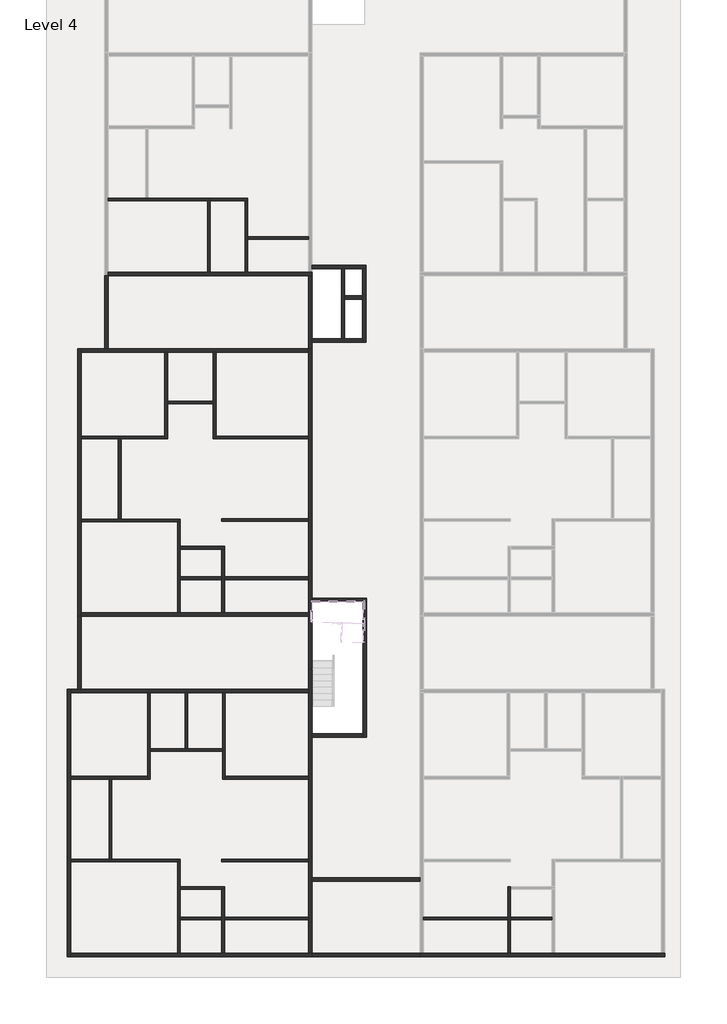
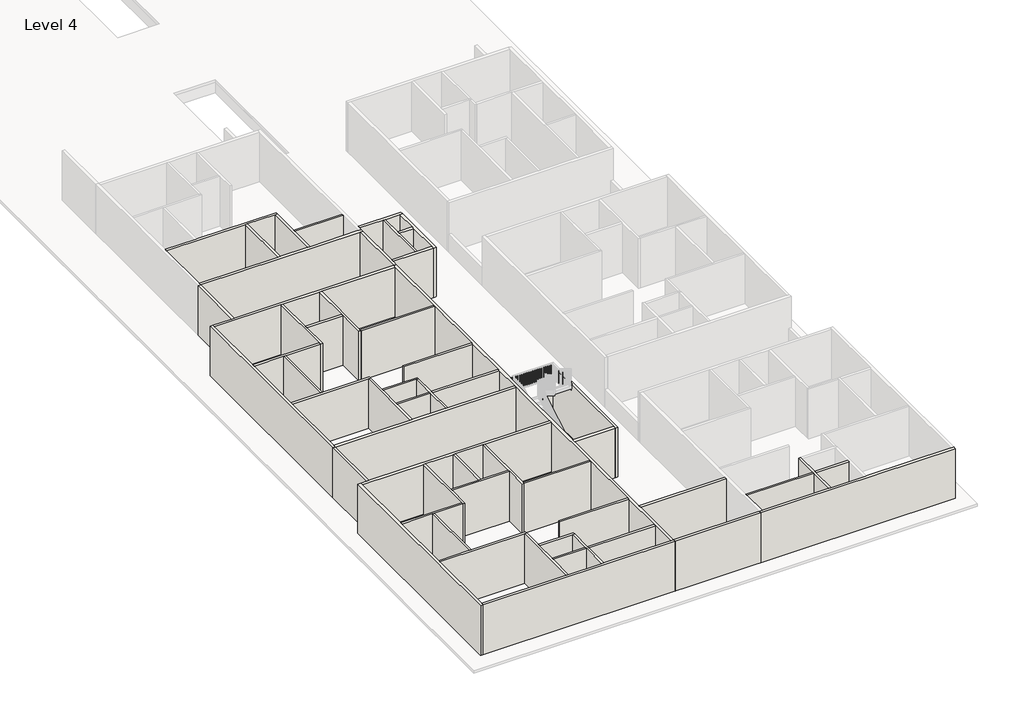
# One storey, part 1 of 8: 55 walls.
"""IFC4 building model written with IfcOpenShell, lengths in millimetres."""

from ifc_helpers import new_model, si_unit, frame, origin, place, context, project, spatial, polyline, outline, extrude, faceted_brep, element, save

model = new_model("IFC4")

# Units and contexts
model_context = context("Model", 3, world=origin())
ifc_project = project(units=[si_unit("LENGTHUNIT", "METRE", prefix="MILLI")], contexts=[model_context])

# Site, building, storey
site = spatial("IfcSite", under=ifc_project)
building = spatial("IfcBuilding", under=site)
storey = spatial("IfcBuildingStorey", under=building, Name="Level 4", Elevation=34378.6172466)

# Walls
placement = place(None, origin())
element("IfcWall", 1, ObjectType="4.5\"", at=placement, inside=storey, context=model_context, shape_type="Brep", body=[
    faceted_brep([(-12531.5544854, -1061.7344126, 34378.6172466), (-8188.1544854, -1061.7344126, 34378.6172466), (-8073.8544854, -1061.7344126, 34378.6172466), (-6549.8544854, -1061.7344126, 34378.6172466), (-6435.5544854, -1061.7344126, 34378.6172466), (-6435.5544854, -1061.7344126, 37426.6172466), (-6549.8544854, -1061.7344126, 37426.6172466), (-8073.8544854, -1061.7344126, 37426.6172466), (-8188.1544854, -1061.7344126, 37426.6172466), (-12531.5544854, -1061.7344126, 37426.6172466), (-12531.5544854, -947.4344126, 34378.6172466), (-12531.5544854, -947.4344126, 37426.6172466), (-10907.2415084, -947.4344126, 37426.6172466), (-10792.9415084, -947.4344126, 37426.6172466), (-6435.5544854, -947.4344126, 37426.6172466), (-6435.5544854, -947.4344126, 34378.6172466), (-10792.9415084, -947.4344126, 34378.6172466), (-10907.2415084, -947.4344126, 34378.6172466)], [[[0, 1, 2, 3, 4, 5, 6, 7, 8, 9]], [[10, 11, 12, 13, 14, 15, 16, 17]], [[4, 3, 2, 1, 0, 10, 17, 16, 15]], [[0, 9, 11, 10]], [[5, 4, 15, 14]], [[9, 8, 7, 6, 5, 14, 13, 12, 11]]]),
])
element("IfcWall", 2, ObjectType="4.5\"", at=placement, inside=storey, context=model_context, shape_type="Brep", body=[
    faceted_brep([(-6549.8544854, -1061.7344126, 34378.6172466), (-6549.8544854, -4185.9344126, 34378.6172466), (-6549.8544854, -4185.9344126, 37426.6172466), (-6549.8544854, -1061.7344126, 37426.6172466), (-6435.5544854, -1061.7344126, 34378.6172466), (-6435.5544854, -1061.7344126, 37426.6172466), (-6435.5544854, -2623.8344126, 37426.6172466), (-6435.5544854, -2738.1344126, 37426.6172466), (-6435.5544854, -4185.9344126, 37426.6172466), (-6435.5544854, -4185.9344126, 34378.6172466), (-6435.5544854, -2738.1344126, 34378.6172466), (-6435.5544854, -2623.8344126, 34378.6172466)], [[[0, 1, 2, 3]], [[4, 5, 6, 7, 8, 9, 10, 11]], [[1, 0, 4, 11, 10, 9]], [[0, 3, 5, 4]], [[2, 1, 9, 8]], [[3, 2, 8, 7, 6, 5]]]),
])
element("IfcWall", 3, ObjectType="4.5\"", at=placement, inside=storey, context=model_context, shape_type="SweptSolid", body=[
    extrude(outline(polyline([(-8188.1544854, -4185.9344126), (-8188.1544854, -1061.7344126), (-8073.8544854, -1061.7344126), (-8073.8544854, -4185.9344126), (-8188.1544854, -4185.9344126)])), frame((0.0, 0.0, 34378.6172466), z_axis=(0.0, 0.0, 1.0), x_axis=(1.0, 0.0, 0.0)), (0.0, 0.0, 1.0), 3048.0),
])
element("IfcWall", 4, ObjectType="4.5\"", at=placement, inside=storey, context=model_context, shape_type="SweptSolid", body=[
    extrude(outline(polyline([(-6435.5544854, -2623.8344126), (-3769.8415084, -2623.8344126), (-3769.8415084, -2738.1344126), (-6435.5544854, -2738.1344126), (-6435.5544854, -2623.8344126)])), frame((0.0, 0.0, 34378.6172466), z_axis=(0.0, 0.0, 1.0), x_axis=(1.0, 0.0, 0.0)), (0.0, 0.0, 1.0), 3048.0),
])
element("IfcWall", 5, ObjectType="4.5\"", at=placement, inside=storey, context=model_context, shape_type="Brep", body=[
    faceted_brep([(-10061.4044854, -7691.1344126, 34378.6172466), (-10061.4044854, -11348.7344126, 34378.6172466), (-10061.4044854, -11463.0344126, 34378.6172466), (-10061.4044854, -11463.0344126, 37426.6172466), (-10061.4044854, -11348.7344126, 37426.6172466), (-10061.4044854, -7691.1344126, 37426.6172466), (-9947.1044854, -7691.1344126, 34378.6172466), (-9947.1044854, -7691.1344126, 37426.6172466), (-9947.1044854, -9824.7344126, 37426.6172466), (-9947.1044854, -9939.0344126, 37426.6172466), (-9947.1044854, -11463.0344126, 37426.6172466), (-9947.1044854, -11463.0344126, 34378.6172466), (-9947.1044854, -9939.0344126, 34378.6172466), (-9947.1044854, -9824.7344126, 34378.6172466)], [[[0, 1, 2, 3, 4, 5]], [[6, 7, 8, 9, 10, 11, 12, 13]], [[2, 1, 0, 6, 13, 12, 11]], [[0, 5, 7, 6]], [[3, 2, 11, 10]], [[5, 4, 3, 10, 9, 8, 7]]]),
])
element("IfcWall", 6, ObjectType="4.5\"", at=placement, inside=storey, context=model_context, shape_type="Brep", body=[
    faceted_brep([(-10061.4044854, -11348.7344126, 34378.6172466), (-13719.0044854, -11348.7344126, 34378.6172466), (-13719.0044854, -11348.7344126, 37426.6172466), (-10061.4044854, -11348.7344126, 37426.6172466), (-10061.4044854, -11463.0344126, 34378.6172466), (-10061.4044854, -11463.0344126, 37426.6172466), (-11980.3915084, -11463.0344126, 37426.6172466), (-12094.6915084, -11463.0344126, 37426.6172466), (-13719.0044854, -11463.0344126, 37426.6172466), (-13719.0044854, -11463.0344126, 34378.6172466), (-12094.6915084, -11463.0344126, 34378.6172466), (-11980.3915084, -11463.0344126, 34378.6172466)], [[[0, 1, 2, 3]], [[4, 5, 6, 7, 8, 9, 10, 11]], [[1, 0, 4, 11, 10, 9]], [[0, 3, 5, 4]], [[2, 1, 9, 8]], [[3, 2, 8, 7, 6, 5]]]),
])
element("IfcWall", 7, ObjectType="4.5\"", at=placement, inside=storey, context=model_context, shape_type="SweptSolid", body=[
    extrude(outline(polyline([(-12094.6915084, -14968.2344126), (-12094.6915084, -11463.0344126), (-11980.3915084, -11463.0344126), (-11980.3915084, -14968.2344126), (-12094.6915084, -14968.2344126)])), frame((0.0, 0.0, 34378.6172466), z_axis=(0.0, 0.0, 1.0), x_axis=(1.0, 0.0, 0.0)), (0.0, 0.0, 1.0), 3048.0),
])
element("IfcWall", 8, ObjectType="4.5\"", at=placement, inside=storey, context=model_context, shape_type="Brep", body=[
    faceted_brep([(-13719.0044854, -15095.2344126, 34378.6172466), (-9510.2415084, -15095.2344126, 34378.6172466), (-9395.9415084, -15095.2344126, 34378.6172466), (-9395.9415084, -15095.2344126, 37426.6172466), (-9510.2415084, -15095.2344126, 37426.6172466), (-13719.0044854, -15095.2344126, 37426.6172466), (-13719.0044854, -14980.9344126, 34378.6172466), (-13719.0044854, -14980.9344126, 37426.6172466), (-9395.9415084, -14980.9344126, 37426.6172466), (-9395.9415084, -14980.9344126, 34378.6172466)], [[[0, 1, 2, 3, 4, 5]], [[6, 7, 8, 9]], [[2, 1, 0, 6, 9]], [[0, 5, 7, 6]], [[3, 2, 9, 8]], [[5, 4, 3, 8, 7]]]),
])
element("IfcWall", 9, ObjectType="4.5\"", at=placement, inside=storey, context=model_context, shape_type="Brep", body=[
    faceted_brep([(-9510.2415084, -15095.2344126, 34378.6172466), (-9510.2415084, -19070.3344126, 34378.6172466), (-9510.2415084, -19070.3344126, 37426.6172466), (-9510.2415084, -15095.2344126, 37426.6172466), (-9395.9415084, -15095.2344126, 34378.6172466), (-9395.9415084, -15095.2344126, 37426.6172466), (-9395.9415084, -16174.7344126, 37426.6172466), (-9395.9415084, -16289.0344126, 37426.6172466), (-9395.9415084, -17508.2344126, 37426.6172466), (-9395.9415084, -17622.5344126, 37426.6172466), (-9395.9415084, -19070.3344126, 37426.6172466), (-9395.9415084, -19070.3344126, 34378.6172466), (-9395.9415084, -17622.5344126, 34378.6172466), (-9395.9415084, -17508.2344126, 34378.6172466), (-9395.9415084, -16289.0344126, 34378.6172466), (-9395.9415084, -16174.7344126, 34378.6172466)], [[[0, 1, 2, 3]], [[4, 5, 6, 7, 8, 9, 10, 11, 12, 13, 14, 15]], [[1, 0, 4, 15, 14, 13, 12, 11]], [[0, 3, 5, 4]], [[2, 1, 11, 10]], [[3, 2, 10, 9, 8, 7, 6, 5]]]),
])
element("IfcWall", 10, ObjectType="4.5\"", at=placement, inside=storey, context=model_context, shape_type="Brep", body=[
    faceted_brep([(-9395.9415084, -16289.0344126, 34378.6172466), (-7567.1415084, -16289.0344126, 34378.6172466), (-7452.8415084, -16289.0344126, 34378.6172466), (-7452.8415084, -16289.0344126, 37426.6172466), (-7567.1415084, -16289.0344126, 37426.6172466), (-9395.9415084, -16289.0344126, 37426.6172466), (-9395.9415084, -16174.7344126, 34378.6172466), (-9395.9415084, -16174.7344126, 37426.6172466), (-7452.8415084, -16174.7344126, 37426.6172466), (-7452.8415084, -16174.7344126, 34378.6172466)], [[[0, 1, 2, 3, 4, 5]], [[6, 7, 8, 9]], [[2, 1, 0, 6, 9]], [[0, 5, 7, 6]], [[3, 2, 9, 8]], [[5, 4, 3, 8, 7]]]),
])
element("IfcWall", 11, ObjectType="4.5\"", at=placement, inside=storey, context=model_context, shape_type="Brep", body=[
    faceted_brep([(-7567.1415084, -16289.0344126, 34378.6172466), (-7567.1415084, -17508.2344126, 34378.6172466), (-7567.1415084, -17622.5344126, 34378.6172466), (-7567.1415084, -19070.3344126, 34378.6172466), (-7567.1415084, -19070.3344126, 37426.6172466), (-7567.1415084, -17622.5344126, 37426.6172466), (-7567.1415084, -17508.2344126, 37426.6172466), (-7567.1415084, -16289.0344126, 37426.6172466), (-7452.8415084, -16289.0344126, 34378.6172466), (-7452.8415084, -16289.0344126, 37426.6172466), (-7452.8415084, -17508.2344126, 37426.6172466), (-7452.8415084, -17622.5344126, 37426.6172466), (-7452.8415084, -19070.3344126, 37426.6172466), (-7452.8415084, -19070.3344126, 34378.6172466), (-7452.8415084, -17622.5344126, 34378.6172466), (-7452.8415084, -17508.2344126, 34378.6172466)], [[[0, 1, 2, 3, 4, 5, 6, 7]], [[8, 9, 10, 11, 12, 13, 14, 15]], [[3, 2, 1, 0, 8, 15, 14, 13]], [[0, 7, 9, 8]], [[4, 3, 13, 12]], [[7, 6, 5, 4, 12, 11, 10, 9]]]),
])
element("IfcWall", 12, ObjectType="4.5\"", at=placement, inside=storey, context=model_context, shape_type="SweptSolid", body=[
    extrude(outline(polyline([(-7567.1415084, -17622.5344126), (-9395.9415084, -17622.5344126), (-9395.9415084, -17508.2344126), (-7567.1415084, -17508.2344126), (-7567.1415084, -17622.5344126)])), frame((0.0, 0.0, 34378.6172466), z_axis=(0.0, 0.0, 1.0), x_axis=(1.0, 0.0, 0.0)), (0.0, 0.0, 1.0), 3048.0),
])
element("IfcWall", 13, ObjectType="4.5\"", at=placement, inside=storey, context=model_context, shape_type="SweptSolid", body=[
    extrude(outline(polyline([(-3769.8415084, -17622.5344126), (-7452.8415084, -17622.5344126), (-7452.8415084, -17508.2344126), (-3769.8415084, -17508.2344126), (-3769.8415084, -17622.5344126)])), frame((0.0, 0.0, 34378.6172466), z_axis=(0.0, 0.0, 1.0), x_axis=(1.0, 0.0, 0.0)), (0.0, 0.0, 1.0), 3048.0),
])
element("IfcWall", 14, ObjectType="4.5\"", at=placement, inside=storey, context=model_context, shape_type="SweptSolid", body=[
    extrude(outline(polyline([(-7567.1415084, -14968.2344126), (-3769.8415084, -14968.2344126), (-3769.8415084, -15082.5344126), (-7567.1415084, -15082.5344126), (-7567.1415084, -14968.2344126)])), frame((0.0, 0.0, 34378.6172466), z_axis=(0.0, 0.0, 1.0), x_axis=(1.0, 0.0, 0.0)), (0.0, 0.0, 1.0), 3048.0),
])
element("IfcWall", 15, ObjectType="4.5\"", at=placement, inside=storey, context=model_context, shape_type="SweptSolid", body=[
    extrude(outline(polyline([(-7940.5044854, -9939.0344126), (-9947.1044854, -9939.0344126), (-9947.1044854, -9824.7344126), (-7940.5044854, -9824.7344126), (-7940.5044854, -9939.0344126)])), frame((0.0, 0.0, 34378.6172466), z_axis=(0.0, 0.0, 1.0), x_axis=(1.0, 0.0, 0.0)), (0.0, 0.0, 1.0), 3048.0),
])
element("IfcWall", 16, ObjectType="4.5\"", at=placement, inside=storey, context=model_context, shape_type="Brep", body=[
    faceted_brep([(-7940.5044854, -7691.1344126, 34378.6172466), (-7940.5044854, -9824.7344126, 34378.6172466), (-7940.5044854, -9939.0344126, 34378.6172466), (-7940.5044854, -11463.0344126, 34378.6172466), (-7940.5044854, -11463.0344126, 37426.6172466), (-7940.5044854, -9939.0344126, 37426.6172466), (-7940.5044854, -9824.7344126, 37426.6172466), (-7940.5044854, -7691.1344126, 37426.6172466), (-7826.2044854, -7691.1344126, 34378.6172466), (-7826.2044854, -7691.1344126, 37426.6172466), (-7826.2044854, -11348.7344126, 37426.6172466), (-7826.2044854, -11463.0344126, 37426.6172466), (-7826.2044854, -11463.0344126, 34378.6172466), (-7826.2044854, -11348.7344126, 34378.6172466)], [[[0, 1, 2, 3, 4, 5, 6, 7]], [[8, 9, 10, 11, 12, 13]], [[3, 2, 1, 0, 8, 13, 12]], [[0, 7, 9, 8]], [[4, 3, 12, 11]], [[7, 6, 5, 4, 11, 10, 9]]]),
])
element("IfcWall", 17, ObjectType="4.5\"", at=placement, inside=storey, context=model_context, shape_type="SweptSolid", body=[
    extrude(outline(polyline([(-3769.8415084, -11463.0344126), (-7826.2044854, -11463.0344126), (-7826.2044854, -11348.7344126), (-3769.8415084, -11348.7344126), (-3769.8415084, -11463.0344126)])), frame((0.0, 0.0, 34378.6172466), z_axis=(0.0, 0.0, 1.0), x_axis=(1.0, 0.0, 0.0)), (0.0, 0.0, 1.0), 3048.0),
])
element("IfcWall", 18, ObjectType="4.5\"", at=placement, inside=storey, context=model_context, shape_type="Brep", body=[
    faceted_brep([(-10818.3415084, -22575.5344126, 34378.6172466), (-10818.3415084, -26233.1344126, 34378.6172466), (-10818.3415084, -26347.4344126, 34378.6172466), (-10818.3415084, -26347.4344126, 37426.6172466), (-10818.3415084, -26233.1344126, 37426.6172466), (-10818.3415084, -22575.5344126, 37426.6172466), (-10704.0415084, -22575.5344126, 34378.6172466), (-10704.0415084, -22575.5344126, 37426.6172466), (-10704.0415084, -25013.9344126, 37426.6172466), (-10704.0415084, -25128.2344126, 37426.6172466), (-10704.0415084, -26347.4344126, 37426.6172466), (-10704.0415084, -26347.4344126, 34378.6172466), (-10704.0415084, -25128.2344126, 34378.6172466), (-10704.0415084, -25013.9344126, 34378.6172466)], [[[0, 1, 2, 3, 4, 5]], [[6, 7, 8, 9, 10, 11, 12, 13]], [[2, 1, 0, 6, 13, 12, 11]], [[0, 5, 7, 6]], [[3, 2, 11, 10]], [[5, 4, 3, 10, 9, 8, 7]]]),
])
element("IfcWall", 19, ObjectType="4.5\"", at=placement, inside=storey, context=model_context, shape_type="Brep", body=[
    faceted_brep([(-10818.3415084, -26233.1344126, 34378.6172466), (-14171.1415084, -26233.1344126, 34378.6172466), (-14171.1415084, -26233.1344126, 37426.6172466), (-10818.3415084, -26233.1344126, 37426.6172466), (-10818.3415084, -26347.4344126, 34378.6172466), (-10818.3415084, -26347.4344126, 37426.6172466), (-12380.4415084, -26347.4344126, 37426.6172466), (-12494.7415084, -26347.4344126, 37426.6172466), (-14171.1415084, -26347.4344126, 37426.6172466), (-14171.1415084, -26347.4344126, 34378.6172466), (-12494.7415084, -26347.4344126, 34378.6172466), (-12380.4415084, -26347.4344126, 34378.6172466)], [[[0, 1, 2, 3]], [[4, 5, 6, 7, 8, 9, 10, 11]], [[1, 0, 4, 11, 10, 9]], [[0, 3, 5, 4]], [[2, 1, 9, 8]], [[3, 2, 8, 7, 6, 5]]]),
])
element("IfcWall", 20, ObjectType="4.5\"", at=placement, inside=storey, context=model_context, shape_type="SweptSolid", body=[
    extrude(outline(polyline([(-9180.0415084, -25013.9344126), (-9180.0415084, -22575.5344126), (-9065.7415084, -22575.5344126), (-9065.7415084, -25013.9344126), (-9180.0415084, -25013.9344126)])), frame((0.0, 0.0, 34378.6172466), z_axis=(0.0, 0.0, 1.0), x_axis=(1.0, 0.0, 0.0)), (0.0, 0.0, 1.0), 3048.0),
])
element("IfcWall", 21, ObjectType="4.5\"", at=placement, inside=storey, context=model_context, shape_type="Brep", body=[
    faceted_brep([(-10704.0415084, -25128.2344126, 34378.6172466), (-7541.7415084, -25128.2344126, 34378.6172466), (-7541.7415084, -25128.2344126, 37426.6172466), (-10704.0415084, -25128.2344126, 37426.6172466), (-10704.0415084, -25013.9344126, 34378.6172466), (-10704.0415084, -25013.9344126, 37426.6172466), (-9180.0415084, -25013.9344126, 37426.6172466), (-9065.7415084, -25013.9344126, 37426.6172466), (-7541.7415084, -25013.9344126, 37426.6172466), (-7541.7415084, -25013.9344126, 34378.6172466), (-9065.7415084, -25013.9344126, 34378.6172466), (-9180.0415084, -25013.9344126, 34378.6172466)], [[[0, 1, 2, 3]], [[4, 5, 6, 7, 8, 9, 10, 11]], [[1, 0, 4, 11, 10, 9]], [[0, 3, 5, 4]], [[2, 1, 9, 8]], [[3, 2, 8, 7, 6, 5]]]),
])
element("IfcWall", 22, ObjectType="4.5\"", at=placement, inside=storey, context=model_context, shape_type="Brep", body=[
    faceted_brep([(-7541.7415084, -22575.5344126, 34378.6172466), (-7541.7415084, -25013.9344126, 34378.6172466), (-7541.7415084, -25128.2344126, 34378.6172466), (-7541.7415084, -26347.4344126, 34378.6172466), (-7541.7415084, -26347.4344126, 37426.6172466), (-7541.7415084, -25128.2344126, 37426.6172466), (-7541.7415084, -25013.9344126, 37426.6172466), (-7541.7415084, -22575.5344126, 37426.6172466), (-7427.4415084, -22575.5344126, 34378.6172466), (-7427.4415084, -22575.5344126, 37426.6172466), (-7427.4415084, -26233.1344126, 37426.6172466), (-7427.4415084, -26347.4344126, 37426.6172466), (-7427.4415084, -26347.4344126, 34378.6172466), (-7427.4415084, -26233.1344126, 34378.6172466)], [[[0, 1, 2, 3, 4, 5, 6, 7]], [[8, 9, 10, 11, 12, 13]], [[3, 2, 1, 0, 8, 13, 12]], [[0, 7, 9, 8]], [[4, 3, 12, 11]], [[7, 6, 5, 4, 11, 10, 9]]]),
])
element("IfcWall", 23, ObjectType="4.5\"", at=placement, inside=storey, context=model_context, shape_type="SweptSolid", body=[
    extrude(outline(polyline([(-3769.8415084, -26347.4344126), (-7427.4415084, -26347.4344126), (-7427.4415084, -26233.1344126), (-3769.8415084, -26233.1344126), (-3769.8415084, -26347.4344126)])), frame((0.0, 0.0, 34378.6172466), z_axis=(0.0, 0.0, 1.0), x_axis=(1.0, 0.0, 0.0)), (0.0, 0.0, 1.0), 3048.0),
])
element("IfcWall", 24, ObjectType="4.5\"", at=placement, inside=storey, context=model_context, shape_type="SweptSolid", body=[
    extrude(outline(polyline([(-12494.7415084, -29852.6344126), (-12494.7415084, -26347.4344126), (-12380.4415084, -26347.4344126), (-12380.4415084, -29852.6344126), (-12494.7415084, -29852.6344126)])), frame((0.0, 0.0, 34378.6172466), z_axis=(0.0, 0.0, 1.0), x_axis=(1.0, 0.0, 0.0)), (0.0, 0.0, 1.0), 3048.0),
])
element("IfcWall", 25, ObjectType="4.5\"", at=placement, inside=storey, context=model_context, shape_type="Brep", body=[
    faceted_brep([(-14171.1415084, -29966.9344126, 34378.6172466), (-9510.2415084, -29966.9344126, 34378.6172466), (-9395.9415084, -29966.9344126, 34378.6172466), (-9395.9415084, -29966.9344126, 37426.6172466), (-9510.2415084, -29966.9344126, 37426.6172466), (-14171.1415084, -29966.9344126, 37426.6172466), (-14171.1415084, -29852.6344126, 34378.6172466), (-14171.1415084, -29852.6344126, 37426.6172466), (-12494.7415084, -29852.6344126, 37426.6172466), (-12380.4415084, -29852.6344126, 37426.6172466), (-9395.9415084, -29852.6344126, 37426.6172466), (-9395.9415084, -29852.6344126, 34378.6172466), (-12380.4415084, -29852.6344126, 34378.6172466), (-12494.7415084, -29852.6344126, 34378.6172466)], [[[0, 1, 2, 3, 4, 5]], [[6, 7, 8, 9, 10, 11, 12, 13]], [[2, 1, 0, 6, 13, 12, 11]], [[0, 5, 7, 6]], [[3, 2, 11, 10]], [[5, 4, 3, 10, 9, 8, 7]]]),
])
element("IfcWall", 26, ObjectType="4.5\"", at=placement, inside=storey, context=model_context, shape_type="Brep", body=[
    faceted_brep([(-9510.2415084, -29966.9344126, 34378.6172466), (-9510.2415084, -33954.7344126, 34378.6172466), (-9510.2415084, -33954.7344126, 37426.6172466), (-9510.2415084, -29966.9344126, 37426.6172466), (-9395.9415084, -29966.9344126, 34378.6172466), (-9395.9415084, -29966.9344126, 37426.6172466), (-9395.9415084, -31059.1344126, 37426.6172466), (-9395.9415084, -31173.4344126, 37426.6172466), (-9395.9415084, -32392.6344126, 37426.6172466), (-9395.9415084, -32506.9344126, 37426.6172466), (-9395.9415084, -33954.7344126, 37426.6172466), (-9395.9415084, -33954.7344126, 34378.6172466), (-9395.9415084, -32506.9344126, 34378.6172466), (-9395.9415084, -32392.6344126, 34378.6172466), (-9395.9415084, -31173.4344126, 34378.6172466), (-9395.9415084, -31059.1344126, 34378.6172466)], [[[0, 1, 2, 3]], [[4, 5, 6, 7, 8, 9, 10, 11, 12, 13, 14, 15]], [[1, 0, 4, 15, 14, 13, 12, 11]], [[0, 3, 5, 4]], [[2, 1, 11, 10]], [[3, 2, 10, 9, 8, 7, 6, 5]]]),
])
element("IfcWall", 27, ObjectType="4.5\"", at=placement, inside=storey, context=model_context, shape_type="Brep", body=[
    faceted_brep([(-9395.9415084, -31173.4344126, 34378.6172466), (-7567.1415084, -31173.4344126, 34378.6172466), (-7452.8415084, -31173.4344126, 34378.6172466), (-7452.8415084, -31173.4344126, 37426.6172466), (-7567.1415084, -31173.4344126, 37426.6172466), (-9395.9415084, -31173.4344126, 37426.6172466), (-9395.9415084, -31059.1344126, 34378.6172466), (-9395.9415084, -31059.1344126, 37426.6172466), (-7452.8415084, -31059.1344126, 37426.6172466), (-7452.8415084, -31059.1344126, 34378.6172466)], [[[0, 1, 2, 3, 4, 5]], [[6, 7, 8, 9]], [[2, 1, 0, 6, 9]], [[0, 5, 7, 6]], [[3, 2, 9, 8]], [[5, 4, 3, 8, 7]]]),
])
element("IfcWall", 28, ObjectType="4.5\"", at=placement, inside=storey, context=model_context, shape_type="Brep", body=[
    faceted_brep([(-7567.1415084, -31173.4344126, 34378.6172466), (-7567.1415084, -32392.6344126, 34378.6172466), (-7567.1415084, -32506.9344126, 34378.6172466), (-7567.1415084, -33954.7344126, 34378.6172466), (-7567.1415084, -33954.7344126, 37426.6172466), (-7567.1415084, -32506.9344126, 37426.6172466), (-7567.1415084, -32392.6344126, 37426.6172466), (-7567.1415084, -31173.4344126, 37426.6172466), (-7452.8415084, -31173.4344126, 34378.6172466), (-7452.8415084, -31173.4344126, 37426.6172466), (-7452.8415084, -32392.6344126, 37426.6172466), (-7452.8415084, -32506.9344126, 37426.6172466), (-7452.8415084, -33954.7344126, 37426.6172466), (-7452.8415084, -33954.7344126, 34378.6172466), (-7452.8415084, -32506.9344126, 34378.6172466), (-7452.8415084, -32392.6344126, 34378.6172466)], [[[0, 1, 2, 3, 4, 5, 6, 7]], [[8, 9, 10, 11, 12, 13, 14, 15]], [[3, 2, 1, 0, 8, 15, 14, 13]], [[0, 7, 9, 8]], [[4, 3, 13, 12]], [[7, 6, 5, 4, 12, 11, 10, 9]]]),
])
element("IfcWall", 29, ObjectType="4.5\"", at=placement, inside=storey, context=model_context, shape_type="SweptSolid", body=[
    extrude(outline(polyline([(-3769.8415084, -32392.6344126), (-3769.8415084, -32506.9344126), (-7452.8415084, -32506.9344126), (-7452.8415084, -32392.6344126), (-3769.8415084, -32392.6344126)])), frame((0.0, 0.0, 34378.6172466), z_axis=(0.0, 0.0, 1.0), x_axis=(1.0, 0.0, 0.0)), (0.0, 0.0, 1.0), 3048.0),
    extrude(outline(polyline([(-9395.9415084, -32506.9344126), (-9395.9415084, -32392.6344126), (-7567.1415084, -32392.6344126), (-7567.1415084, -32506.9344126), (-9395.9415084, -32506.9344126)])), frame((0.0, 0.0, 34378.6172466), z_axis=(0.0, 0.0, 1.0), x_axis=(1.0, 0.0, 0.0)), (0.0, 0.0, 1.0), 3048.0),
])
element("IfcWall", 30, ObjectType="4.5\"", at=placement, inside=storey, context=model_context, shape_type="SweptSolid", body=[
    extrude(outline(polyline([(-7567.1415084, -29852.6344126), (-3769.8415084, -29852.6344126), (-3769.8415084, -29966.9344126), (-7567.1415084, -29966.9344126), (-7567.1415084, -29852.6344126)])), frame((0.0, 0.0, 34378.6172466), z_axis=(0.0, 0.0, 1.0), x_axis=(1.0, 0.0, 0.0)), (0.0, 0.0, 1.0), 3048.0),
])
element("IfcWall", 31, ObjectType="4.5\"", at=placement, inside=storey, context=model_context, shape_type="SweptSolid", body=[
    extrude(outline(polyline([(4942.3584916, -32506.9344126), (1259.3584916, -32506.9344126), (1259.3584916, -32392.6344126), (4942.3584916, -32392.6344126), (4942.3584916, -32506.9344126)])), frame((0.0, 0.0, 34378.6172466), z_axis=(0.0, 0.0, 1.0), x_axis=(1.0, 0.0, 0.0)), (0.0, 0.0, 1.0), 3048.0),
])
element("IfcWall", 32, ObjectType="4.5\"", at=placement, inside=storey, context=model_context, shape_type="Brep", body=[
    faceted_brep([(4942.3584916, -31059.1344126, 34378.6172466), (4942.3584916, -32392.6344126, 34378.6172466), (4942.3584916, -32506.9344126, 34378.6172466), (4942.3584916, -33954.7344126, 34378.6172466), (4942.3584916, -33954.7344126, 37426.6172466), (4942.3584916, -32506.9344126, 37426.6172466), (4942.3584916, -32392.6344126, 37426.6172466), (4942.3584916, -31059.1344126, 37426.6172466), (5056.6584916, -31059.1344126, 34378.6172466), (5056.6584916, -31059.1344126, 37426.6172466), (5056.6584916, -31173.4344126, 37426.6172466), (5056.6584916, -32392.6344126, 37426.6172466), (5056.6584916, -32506.9344126, 37426.6172466), (5056.6584916, -33954.7344126, 37426.6172466), (5056.6584916, -33954.7344126, 34378.6172466), (5056.6584916, -32506.9344126, 34378.6172466), (5056.6584916, -32392.6344126, 34378.6172466), (5056.6584916, -31173.4344126, 34378.6172466)], [[[0, 1, 2, 3, 4, 5, 6, 7]], [[8, 9, 10, 11, 12, 13, 14, 15, 16, 17]], [[3, 2, 1, 0, 8, 17, 16, 15, 14]], [[4, 3, 14, 13]], [[0, 7, 9, 8]], [[7, 6, 5, 4, 13, 12, 11, 10, 9]]]),
])
element("IfcWall", 33, ObjectType="4.5\"", at=placement, inside=storey, context=model_context, shape_type="SweptSolid", body=[
    extrude(outline(polyline([(6885.4584916, -32506.9344126), (5056.6584916, -32506.9344126), (5056.6584916, -32392.6344126), (6885.4584916, -32392.6344126), (6885.4584916, -32506.9344126)])), frame((0.0, 0.0, 34378.6172466), z_axis=(0.0, 0.0, 1.0), x_axis=(1.0, 0.0, 0.0)), (0.0, 0.0, 1.0), 3048.0),
])
element("IfcWall", 34, ObjectType="4.5\"", at=placement, inside=storey, context=model_context, shape_type="Brep", body=[
    faceted_brep([(-2207.6738684, -7082.6751812, 34378.6172466), (-2207.6738684, -5366.3479894, 34378.6172466), (-2207.6738684, -5213.9479894, 34378.6172466), (-2207.6738684, -4034.6751812, 34378.6172466), (-2207.6738684, -4034.6751812, 37426.6172466), (-2207.6738684, -5213.9479894, 37426.6172466), (-2207.6738684, -5366.3479894, 37426.6172466), (-2207.6738684, -7082.6751812, 37426.6172466), (-2321.9738684, -7082.6751812, 34378.6172466), (-2321.9738684, -7082.6751812, 37426.6172466), (-2321.9738684, -4034.6751812, 37426.6172466), (-2321.9738684, -4034.6751812, 34378.6172466)], [[[0, 1, 2, 3, 4, 5, 6, 7]], [[8, 9, 10, 11]], [[3, 2, 1, 0, 8, 11]], [[7, 6, 5, 4, 10, 9]], [[4, 3, 11, 10]], [[0, 7, 9, 8]]]),
])
element("IfcWall", 35, ObjectType="6\"", at=placement, inside=storey, context=model_context, shape_type="Brep", body=[
    faceted_brep([(-12531.5544854, -4338.3344126, 34378.6172466), (-3769.8415084, -4338.3344126, 34378.6172466), (-3617.4415084, -4338.3344126, 34378.6172466), (-3617.4415084, -4338.3344126, 37426.6172466), (-3769.8415084, -4338.3344126, 37426.6172466), (-12531.5544854, -4338.3344126, 37426.6172466), (-12531.5544854, -4185.9344126, 34378.6172466), (-12531.5544854, -4185.9344126, 37426.6172466), (-8188.1544854, -4185.9344126, 37426.6172466), (-8073.8544854, -4185.9344126, 37426.6172466), (-6549.8544854, -4185.9344126, 37426.6172466), (-6435.5544854, -4185.9344126, 37426.6172466), (-3769.8415084, -4185.9344126, 37426.6172466), (-3617.4415084, -4185.9344126, 37426.6172466), (-3617.4415084, -4185.9344126, 34378.6172466), (-3769.8415084, -4185.9344126, 34378.6172466), (-6435.5544854, -4185.9344126, 34378.6172466), (-6549.8544854, -4185.9344126, 34378.6172466), (-8073.8544854, -4185.9344126, 34378.6172466), (-8188.1544854, -4185.9344126, 34378.6172466)], [[[0, 1, 2, 3, 4, 5]], [[6, 7, 8, 9, 10, 11, 12, 13, 14, 15, 16, 17, 18, 19]], [[2, 1, 0, 6, 19, 18, 17, 16, 15, 14]], [[0, 5, 7, 6]], [[3, 2, 14, 13]], [[5, 4, 3, 13, 12, 11, 10, 9, 8, 7]]]),
])
element("IfcWall", 36, ObjectType="6\"", at=placement, inside=storey, context=model_context, shape_type="Brep", body=[
    faceted_brep([(-13871.4044854, -7538.7344126, 34378.6172466), (-13871.4044854, -19222.7344126, 34378.6172466), (-13871.4044854, -19222.7344126, 37426.6172466), (-13871.4044854, -7538.7344126, 37426.6172466), (-13719.0044854, -7538.7344126, 34378.6172466), (-13719.0044854, -7538.7344126, 37426.6172466), (-13719.0044854, -7691.1344126, 37426.6172466), (-13719.0044854, -11348.7344126, 37426.6172466), (-13719.0044854, -11463.0344126, 37426.6172466), (-13719.0044854, -14980.9344126, 37426.6172466), (-13719.0044854, -15095.2344126, 37426.6172466), (-13719.0044854, -19070.3344126, 37426.6172466), (-13719.0044854, -19222.7344126, 37426.6172466), (-13719.0044854, -19222.7344126, 34378.6172466), (-13719.0044854, -19070.3344126, 34378.6172466), (-13719.0044854, -15095.2344126, 34378.6172466), (-13719.0044854, -14980.9344126, 34378.6172466), (-13719.0044854, -11463.0344126, 34378.6172466), (-13719.0044854, -11348.7344126, 34378.6172466), (-13719.0044854, -7691.1344126, 34378.6172466)], [[[0, 1, 2, 3]], [[4, 5, 6, 7, 8, 9, 10, 11, 12, 13, 14, 15, 16, 17, 18, 19]], [[1, 0, 4, 19, 18, 17, 16, 15, 14, 13]], [[2, 1, 13, 12]], [[0, 3, 5, 4]], [[3, 2, 12, 11, 10, 9, 8, 7, 6, 5]]]),
])
element("IfcWall", 37, ObjectType="6\"", at=placement, inside=storey, context=model_context, shape_type="Brep", body=[
    faceted_brep([(-13719.0044854, -19222.7344126, 34378.6172466), (-3769.8415084, -19222.7344126, 34378.6172466), (-3769.8415084, -19222.7344126, 37426.6172466), (-13719.0044854, -19222.7344126, 37426.6172466), (-13719.0044854, -19070.3344126, 34378.6172466), (-13719.0044854, -19070.3344126, 37426.6172466), (-9510.2415084, -19070.3344126, 37426.6172466), (-9395.9415084, -19070.3344126, 37426.6172466), (-7567.1415084, -19070.3344126, 37426.6172466), (-7452.8415084, -19070.3344126, 37426.6172466), (-3769.8415084, -19070.3344126, 37426.6172466), (-3769.8415084, -19070.3344126, 34378.6172466), (-7452.8415084, -19070.3344126, 34378.6172466), (-7567.1415084, -19070.3344126, 34378.6172466), (-9395.9415084, -19070.3344126, 34378.6172466), (-9510.2415084, -19070.3344126, 34378.6172466)], [[[0, 1, 2, 3]], [[4, 5, 6, 7, 8, 9, 10, 11, 12, 13, 14, 15]], [[1, 0, 4, 15, 14, 13, 12, 11]], [[0, 3, 5, 4]], [[2, 1, 11, 10]], [[3, 2, 10, 9, 8, 7, 6, 5]]]),
])
element("IfcWall", 38, ObjectType="6\"", at=placement, inside=storey, context=model_context, shape_type="Brep", body=[
    faceted_brep([(-3617.4415084, -33954.7344126, 34378.6172466), (-3617.4415084, -30820.9325185, 34378.6172466), (-3617.4415084, -30668.5325185, 34378.6172466), (-3617.4415084, -24525.9851539, 34378.6172466), (-3617.4415084, -24373.5851539, 34378.6172466), (-3617.4415084, -18582.3851539, 34378.6172466), (-3617.4415084, -18429.9851539, 34378.6172466), (-3617.4415084, -7538.7344126, 34378.6172466), (-3617.4415084, -7538.7344126, 37426.6172466), (-3617.4415084, -18429.9851539, 37426.6172466), (-3617.4415084, -18582.3851539, 37426.6172466), (-3617.4415084, -24373.5851539, 37426.6172466), (-3617.4415084, -24525.9851539, 37426.6172466), (-3617.4415084, -30668.5325185, 37426.6172466), (-3617.4415084, -30820.9325185, 37426.6172466), (-3617.4415084, -33954.7344126, 37426.6172466), (-3769.8415084, -33954.7344126, 34378.6172466), (-3769.8415084, -33954.7344126, 37426.6172466), (-3769.8415084, -32506.9344126, 37426.6172466), (-3769.8415084, -32392.6344126, 37426.6172466), (-3769.8415084, -29966.9344126, 37426.6172466), (-3769.8415084, -29852.6344126, 37426.6172466), (-3769.8415084, -26347.4344126, 37426.6172466), (-3769.8415084, -26233.1344126, 37426.6172466), (-3769.8415084, -22575.5344126, 37426.6172466), (-3769.8415084, -22423.1344126, 37426.6172466), (-3769.8415084, -19222.7344126, 37426.6172466), (-3769.8415084, -19070.3344126, 37426.6172466), (-3769.8415084, -17622.5344126, 37426.6172466), (-3769.8415084, -17508.2344126, 37426.6172466), (-3769.8415084, -15082.5344126, 37426.6172466), (-3769.8415084, -14968.2344126, 37426.6172466), (-3769.8415084, -11463.0344126, 37426.6172466), (-3769.8415084, -11348.7344126, 37426.6172466), (-3769.8415084, -7691.1344126, 37426.6172466), (-3769.8415084, -7538.7344126, 37426.6172466), (-3769.8415084, -7538.7344126, 34378.6172466), (-3769.8415084, -7691.1344126, 34378.6172466), (-3769.8415084, -11348.7344126, 34378.6172466), (-3769.8415084, -11463.0344126, 34378.6172466), (-3769.8415084, -14968.2344126, 34378.6172466), (-3769.8415084, -15082.5344126, 34378.6172466), (-3769.8415084, -17508.2344126, 34378.6172466), (-3769.8415084, -17622.5344126, 34378.6172466), (-3769.8415084, -19070.3344126, 34378.6172466), (-3769.8415084, -19222.7344126, 34378.6172466), (-3769.8415084, -22423.1344126, 34378.6172466), (-3769.8415084, -22575.5344126, 34378.6172466), (-3769.8415084, -26233.1344126, 34378.6172466), (-3769.8415084, -26347.4344126, 34378.6172466), (-3769.8415084, -29852.6344126, 34378.6172466), (-3769.8415084, -29966.9344126, 34378.6172466), (-3769.8415084, -32392.6344126, 34378.6172466), (-3769.8415084, -32506.9344126, 34378.6172466)], [[[0, 1, 2, 3, 4, 5, 6, 7, 8, 9, 10, 11, 12, 13, 14, 15]], [[16, 17, 18, 19, 20, 21, 22, 23, 24, 25, 26, 27, 28, 29, 30, 31, 32, 33, 34, 35, 36, 37, 38, 39, 40, 41, 42, 43, 44, 45, 46, 47, 48, 49, 50, 51, 52, 53]], [[7, 6, 5, 4, 3, 2, 1, 0, 16, 53, 52, 51, 50, 49, 48, 47, 46, 45, 44, 43, 42, 41, 40, 39, 38, 37, 36]], [[8, 7, 36, 35]], [[0, 15, 17, 16]], [[15, 14, 13, 12, 11, 10, 9, 8, 35, 34, 33, 32, 31, 30, 29, 28, 27, 26, 25, 24, 23, 22, 21, 20, 19, 18, 17]]]),
])
element("IfcWall", 39, ObjectType="6\"", at=placement, inside=storey, context=model_context, shape_type="Brep", body=[
    faceted_brep([(-3769.8415084, -7538.7344126, 34378.6172466), (-12531.5544854, -7538.7344126, 34378.6172466), (-12683.9544854, -7538.7344126, 34378.6172466), (-13719.0044854, -7538.7344126, 34378.6172466), (-13719.0044854, -7538.7344126, 37426.6172466), (-12683.9544854, -7538.7344126, 37426.6172466), (-12531.5544854, -7538.7344126, 37426.6172466), (-3769.8415084, -7538.7344126, 37426.6172466), (-3769.8415084, -7691.1344126, 34378.6172466), (-3769.8415084, -7691.1344126, 37426.6172466), (-7826.2044854, -7691.1344126, 37426.6172466), (-7940.5044854, -7691.1344126, 37426.6172466), (-9947.1044854, -7691.1344126, 37426.6172466), (-10061.4044854, -7691.1344126, 37426.6172466), (-13719.0044854, -7691.1344126, 37426.6172466), (-13719.0044854, -7691.1344126, 34378.6172466), (-10061.4044854, -7691.1344126, 34378.6172466), (-9947.1044854, -7691.1344126, 34378.6172466), (-7940.5044854, -7691.1344126, 34378.6172466), (-7826.2044854, -7691.1344126, 34378.6172466)], [[[0, 1, 2, 3, 4, 5, 6, 7]], [[8, 9, 10, 11, 12, 13, 14, 15, 16, 17, 18, 19]], [[3, 2, 1, 0, 8, 19, 18, 17, 16, 15]], [[0, 7, 9, 8]], [[4, 3, 15, 14]], [[7, 6, 5, 4, 14, 13, 12, 11, 10, 9]]]),
])
element("IfcWall", 40, ObjectType="6\"", at=placement, inside=storey, context=model_context, shape_type="Brep", body=[
    faceted_brep([(-14323.5415084, -22423.1344126, 34378.6172466), (-14323.5415084, -34107.1344126, 34378.6172466), (-14323.5415084, -34107.1344126, 37426.6172466), (-14323.5415084, -22423.1344126, 37426.6172466), (-14171.1415084, -22423.1344126, 34378.6172466), (-14171.1415084, -22423.1344126, 37426.6172466), (-14171.1415084, -22575.5344126, 37426.6172466), (-14171.1415084, -26233.1344126, 37426.6172466), (-14171.1415084, -26347.4344126, 37426.6172466), (-14171.1415084, -29852.6344126, 37426.6172466), (-14171.1415084, -29966.9344126, 37426.6172466), (-14171.1415084, -33954.7344126, 37426.6172466), (-14171.1415084, -34107.1344126, 37426.6172466), (-14171.1415084, -34107.1344126, 34378.6172466), (-14171.1415084, -33954.7344126, 34378.6172466), (-14171.1415084, -29966.9344126, 34378.6172466), (-14171.1415084, -29852.6344126, 34378.6172466), (-14171.1415084, -26347.4344126, 34378.6172466), (-14171.1415084, -26233.1344126, 34378.6172466), (-14171.1415084, -22575.5344126, 34378.6172466)], [[[0, 1, 2, 3]], [[4, 5, 6, 7, 8, 9, 10, 11, 12, 13, 14, 15, 16, 17, 18, 19]], [[1, 0, 4, 19, 18, 17, 16, 15, 14, 13]], [[2, 1, 13, 12]], [[0, 3, 5, 4]], [[3, 2, 12, 11, 10, 9, 8, 7, 6, 5]]]),
])
element("IfcWall", 41, ObjectType="6\"", at=placement, inside=storey, context=model_context, shape_type="Brep", body=[
    faceted_brep([(-14171.1415084, -34107.1344126, 34378.6172466), (-3617.4415084, -34107.1344126, 34378.6172466), (-3617.4415084, -34107.1344126, 37426.6172466), (-14171.1415084, -34107.1344126, 37426.6172466), (-14171.1415084, -33954.7344126, 34378.6172466), (-14171.1415084, -33954.7344126, 37426.6172466), (-9510.2415084, -33954.7344126, 37426.6172466), (-9395.9415084, -33954.7344126, 37426.6172466), (-7567.1415084, -33954.7344126, 37426.6172466), (-7452.8415084, -33954.7344126, 37426.6172466), (-3769.8415084, -33954.7344126, 37426.6172466), (-3617.4415084, -33954.7344126, 37426.6172466), (-3617.4415084, -33954.7344126, 34378.6172466), (-3769.8415084, -33954.7344126, 34378.6172466), (-7452.8415084, -33954.7344126, 34378.6172466), (-7567.1415084, -33954.7344126, 34378.6172466), (-9395.9415084, -33954.7344126, 34378.6172466), (-9510.2415084, -33954.7344126, 34378.6172466)], [[[0, 1, 2, 3]], [[4, 5, 6, 7, 8, 9, 10, 11, 12, 13, 14, 15, 16, 17]], [[1, 0, 4, 17, 16, 15, 14, 13, 12]], [[0, 3, 5, 4]], [[2, 1, 12, 11]], [[3, 2, 11, 10, 9, 8, 7, 6, 5]]]),
])
element("IfcWall", 42, ObjectType="6\"", at=placement, inside=storey, context=model_context, shape_type="Brep", body=[
    faceted_brep([(-3769.8415084, -22423.1344126, 34378.6172466), (-13719.0044854, -22423.1344126, 34378.6172466), (-13871.4044854, -22423.1344126, 34378.6172466), (-14171.1415084, -22423.1344126, 34378.6172466), (-14171.1415084, -22423.1344126, 37426.6172466), (-13871.4044854, -22423.1344126, 37426.6172466), (-13719.0044854, -22423.1344126, 37426.6172466), (-3769.8415084, -22423.1344126, 37426.6172466), (-3769.8415084, -22575.5344126, 34378.6172466), (-3769.8415084, -22575.5344126, 37426.6172466), (-7427.4415084, -22575.5344126, 37426.6172466), (-7541.7415084, -22575.5344126, 37426.6172466), (-9065.7415084, -22575.5344126, 37426.6172466), (-9180.0415084, -22575.5344126, 37426.6172466), (-10704.0415084, -22575.5344126, 37426.6172466), (-10818.3415084, -22575.5344126, 37426.6172466), (-14171.1415084, -22575.5344126, 37426.6172466), (-14171.1415084, -22575.5344126, 34378.6172466), (-10818.3415084, -22575.5344126, 34378.6172466), (-10704.0415084, -22575.5344126, 34378.6172466), (-9180.0415084, -22575.5344126, 34378.6172466), (-9065.7415084, -22575.5344126, 34378.6172466), (-7541.7415084, -22575.5344126, 34378.6172466), (-7427.4415084, -22575.5344126, 34378.6172466)], [[[0, 1, 2, 3, 4, 5, 6, 7]], [[8, 9, 10, 11, 12, 13, 14, 15, 16, 17, 18, 19, 20, 21, 22, 23]], [[3, 2, 1, 0, 8, 23, 22, 21, 20, 19, 18, 17]], [[0, 7, 9, 8]], [[4, 3, 17, 16]], [[7, 6, 5, 4, 16, 15, 14, 13, 12, 11, 10, 9]]]),
])
element("IfcWall", 43, ObjectType="6\"", at=placement, inside=storey, context=model_context, shape_type="Brep", body=[
    faceted_brep([(1106.9584916, -34107.1344126, 34378.6172466), (11813.0584916, -34107.1344126, 34378.6172466), (11813.0584916, -34107.1344126, 37426.6172466), (1106.9584916, -34107.1344126, 37426.6172466), (1106.9584916, -33954.7344126, 34378.6172466), (1106.9584916, -33954.7344126, 37426.6172466), (1259.3584916, -33954.7344126, 37426.6172466), (4942.3584916, -33954.7344126, 37426.6172466), (5056.6584916, -33954.7344126, 37426.6172466), (6885.4584916, -33954.7344126, 37426.6172466), (6999.7584916, -33954.7344126, 37426.6172466), (11660.6584916, -33954.7344126, 37426.6172466), (11813.0584916, -33954.7344126, 37426.6172466), (11813.0584916, -33954.7344126, 34378.6172466), (11660.6584916, -33954.7344126, 34378.6172466), (6999.7584916, -33954.7344126, 34378.6172466), (6885.4584916, -33954.7344126, 34378.6172466), (5056.6584916, -33954.7344126, 34378.6172466), (4942.3584916, -33954.7344126, 34378.6172466), (1259.3584916, -33954.7344126, 34378.6172466)], [[[0, 1, 2, 3]], [[4, 5, 6, 7, 8, 9, 10, 11, 12, 13, 14, 15, 16, 17, 18, 19]], [[1, 0, 4, 19, 18, 17, 16, 15, 14, 13]], [[2, 1, 13, 12]], [[0, 3, 5, 4]], [[3, 2, 12, 11, 10, 9, 8, 7, 6, 5]]]),
])
element("IfcWall", 44, ObjectType="6\"", at=placement, inside=storey, context=model_context, shape_type="Brep", body=[
    faceted_brep([(-3617.4415084, -18582.3851539, 34378.6172466), (-1382.2415084, -18582.3851539, 34378.6172466), (-1229.8415084, -18582.3851539, 34378.6172466), (-1229.8415084, -18582.3851539, 37426.6172466), (-1382.2415084, -18582.3851539, 37426.6172466), (-3617.4415084, -18582.3851539, 37426.6172466), (-3617.4415084, -18429.9851539, 34378.6172466), (-3617.4415084, -18429.9851539, 37426.6172466), (-1229.8415084, -18429.9851539, 37426.6172466), (-1229.8415084, -18429.9851539, 34378.6172466)], [[[0, 1, 2, 3, 4, 5]], [[6, 7, 8, 9]], [[2, 1, 0, 6, 9]], [[5, 4, 3, 8, 7]], [[0, 5, 7, 6]], [[3, 2, 9, 8]]]),
])
element("IfcWall", 45, ObjectType="6\"", at=placement, inside=storey, context=model_context, shape_type="Brep", body=[
    faceted_brep([(-1382.2415084, -18582.3851539, 34378.6172466), (-1382.2415084, -24373.5851539, 34378.6172466), (-1382.2415084, -24525.9851539, 34378.6172466), (-1382.2415084, -24525.9851539, 37426.6172466), (-1382.2415084, -24373.5851539, 37426.6172466), (-1382.2415084, -18582.3851539, 37426.6172466), (-1229.8415084, -18582.3851539, 34378.6172466), (-1229.8415084, -18582.3851539, 37426.6172466), (-1229.8415084, -24525.9851539, 37426.6172466), (-1229.8415084, -24525.9851539, 34378.6172466)], [[[0, 1, 2, 3, 4, 5]], [[6, 7, 8, 9]], [[2, 1, 0, 6, 9]], [[5, 4, 3, 8, 7]], [[0, 5, 7, 6]], [[3, 2, 9, 8]]]),
])
element("IfcWall", 46, ObjectType="6\"", at=placement, inside=storey, context=model_context, shape_type="SweptSolid", body=[
    extrude(outline(polyline([(-3617.4415084, -24373.5851539), (-1382.2415084, -24373.5851539), (-1382.2415084, -24525.9851539), (-3617.4415084, -24525.9851539), (-3617.4415084, -24373.5851539)])), frame((0.0, 0.0, 34378.6172466), z_axis=(0.0, 0.0, 1.0), x_axis=(1.0, 0.0, 0.0)), (0.0, 0.0, 1.0), 3048.0),
])
element("IfcWall", 47, ObjectType="6\"", at=placement, inside=storey, context=model_context, shape_type="Brep", body=[
    faceted_brep([(-3769.8415084, -4338.3344126, 34378.6172466), (-3769.8415084, -7538.7344126, 34378.6172466), (-3769.8415084, -7538.7344126, 37426.6172466), (-3769.8415084, -4338.3344126, 37426.6172466), (-3617.4415084, -4338.3344126, 34378.6172466), (-3617.4415084, -4338.3344126, 37426.6172466), (-3617.4415084, -7082.6751812, 37426.6172466), (-3617.4415084, -7235.0751812, 37426.6172466), (-3617.4415084, -7538.7344126, 37426.6172466), (-3617.4415084, -7538.7344126, 34378.6172466), (-3617.4415084, -7235.0751812, 34378.6172466), (-3617.4415084, -7082.6751812, 34378.6172466)], [[[0, 1, 2, 3]], [[4, 5, 6, 7, 8, 9, 10, 11]], [[1, 0, 4, 11, 10, 9]], [[0, 3, 5, 4]], [[2, 1, 9, 8]], [[3, 2, 8, 7, 6, 5]]]),
])
element("IfcWall", 48, ObjectType="6\"", at=placement, inside=storey, context=model_context, shape_type="Brep", body=[
    faceted_brep([(-3617.4415084, -4034.6751812, 34378.6172466), (-2321.9738684, -4034.6751812, 34378.6172466), (-2207.6738684, -4034.6751812, 34378.6172466), (-1407.6415084, -4034.6751812, 34378.6172466), (-1255.2415084, -4034.6751812, 34378.6172466), (-1255.2415084, -4034.6751812, 37426.6172466), (-1407.6415084, -4034.6751812, 37426.6172466), (-2207.6738684, -4034.6751812, 37426.6172466), (-2321.9738684, -4034.6751812, 37426.6172466), (-3617.4415084, -4034.6751812, 37426.6172466), (-3617.4415084, -3882.2751812, 34378.6172466), (-3617.4415084, -3882.2751812, 37426.6172466), (-1255.2415084, -3882.2751812, 37426.6172466), (-1255.2415084, -3882.2751812, 34378.6172466)], [[[0, 1, 2, 3, 4, 5, 6, 7, 8, 9]], [[10, 11, 12, 13]], [[4, 3, 2, 1, 0, 10, 13]], [[9, 8, 7, 6, 5, 12, 11]], [[0, 9, 11, 10]], [[5, 4, 13, 12]]]),
])
element("IfcWall", 49, ObjectType="6\"", at=placement, inside=storey, context=model_context, shape_type="Brep", body=[
    faceted_brep([(-1407.6415084, -4034.6751812, 34378.6172466), (-1407.6415084, -5213.9479894, 34378.6172466), (-1407.6415084, -5366.3479894, 34378.6172466), (-1407.6415084, -7082.6751812, 34378.6172466), (-1407.6415084, -7235.0751812, 34378.6172466), (-1407.6415084, -7235.0751812, 37426.6172466), (-1407.6415084, -7082.6751812, 37426.6172466), (-1407.6415084, -5366.3479894, 37426.6172466), (-1407.6415084, -5213.9479894, 37426.6172466), (-1407.6415084, -4034.6751812, 37426.6172466), (-1255.2415084, -4034.6751812, 34378.6172466), (-1255.2415084, -4034.6751812, 37426.6172466), (-1255.2415084, -7235.0751812, 37426.6172466), (-1255.2415084, -7235.0751812, 34378.6172466)], [[[0, 1, 2, 3, 4, 5, 6, 7, 8, 9]], [[10, 11, 12, 13]], [[4, 3, 2, 1, 0, 10, 13]], [[9, 8, 7, 6, 5, 12, 11]], [[0, 9, 11, 10]], [[5, 4, 13, 12]]]),
])
element("IfcWall", 50, ObjectType="6\"", at=placement, inside=storey, context=model_context, shape_type="Brep", body=[
    faceted_brep([(-1407.6415084, -7082.6751812, 34378.6172466), (-2207.6738684, -7082.6751812, 34378.6172466), (-2321.9738684, -7082.6751812, 34378.6172466), (-3617.4415084, -7082.6751812, 34378.6172466), (-3617.4415084, -7082.6751812, 37426.6172466), (-2321.9738684, -7082.6751812, 37426.6172466), (-2207.6738684, -7082.6751812, 37426.6172466), (-1407.6415084, -7082.6751812, 37426.6172466), (-1407.6415084, -7235.0751812, 34378.6172466), (-1407.6415084, -7235.0751812, 37426.6172466), (-3617.4415084, -7235.0751812, 37426.6172466), (-3617.4415084, -7235.0751812, 34378.6172466)], [[[0, 1, 2, 3, 4, 5, 6, 7]], [[8, 9, 10, 11]], [[3, 2, 1, 0, 8, 11]], [[7, 6, 5, 4, 10, 9]], [[0, 7, 9, 8]], [[4, 3, 11, 10]]]),
])
element("IfcWall", 51, ObjectType="6\"", at=placement, inside=storey, context=model_context, shape_type="SweptSolid", body=[
    extrude(outline(polyline([(-2207.6738684, -5213.9479894), (-1407.6415084, -5213.9479894), (-1407.6415084, -5366.3479894), (-2207.6738684, -5366.3479894), (-2207.6738684, -5213.9479894)])), frame((0.0, 0.0, 34378.6172466), z_axis=(0.0, 0.0, 1.0), x_axis=(1.0, 0.0, 0.0)), (0.0, 0.0, 1.0), 3048.0),
])
element("IfcWall", 52, ObjectType="6\" 2", at=placement, inside=storey, context=model_context, shape_type="SweptSolid", body=[
    extrude(outline(polyline([(1106.9584916, -34107.1344126), (-3617.4415084, -34107.1344126), (-3617.4415084, -33954.7344126), (1106.9584916, -33954.7344126), (1106.9584916, -34107.1344126)])), frame((0.0, 0.0, 34378.6172466), z_axis=(0.0, 0.0, 1.0), x_axis=(1.0, 0.0, 0.0)), (0.0, 0.0, 1.0), 3048.0),
])
element("IfcWall", 53, ObjectType="6\" 2", at=placement, inside=storey, context=model_context, shape_type="SweptSolid", body=[
    extrude(outline(polyline([(-3617.4415084, -30668.5325185), (1106.9584916, -30668.5325185), (1106.9584916, -30820.9325185), (-3617.4415084, -30820.9325185), (-3617.4415084, -30668.5325185)])), frame((0.0, 0.0, 34378.6172466), z_axis=(0.0, 0.0, 1.0), x_axis=(1.0, 0.0, 0.0)), (0.0, 0.0, 1.0), 3048.0),
])
element("IfcWall", 54, ObjectType="6\" 2", at=placement, inside=storey, context=model_context, shape_type="SweptSolid", body=[
    extrude(outline(polyline([(-13871.4044854, -22423.1344126), (-13871.4044854, -19222.7344126), (-13719.0044854, -19222.7344126), (-13719.0044854, -22423.1344126), (-13871.4044854, -22423.1344126)])), frame((0.0, 0.0, 34378.6172466), z_axis=(0.0, 0.0, 1.0), x_axis=(1.0, 0.0, 0.0)), (0.0, 0.0, 1.0), 3048.0),
])
element("IfcWall", 55, ObjectType="6\" 2", at=placement, inside=storey, context=model_context, shape_type="SweptSolid", body=[
    extrude(outline(polyline([(-12683.9544854, -7538.7344126), (-12683.9544854, -4338.3344126), (-12531.5544854, -4338.3344126), (-12531.5544854, -7538.7344126), (-12683.9544854, -7538.7344126)])), frame((0.0, 0.0, 34378.6172466), z_axis=(0.0, 0.0, 1.0), x_axis=(1.0, 0.0, 0.0)), (0.0, 0.0, 1.0), 3048.0),
])

save(model, "model.ifc")

# Revit data of these elements
# Type "4.5\""
#   Assembly Code = "B2010"
#   Layers, outside or top first: 0' - 4 1/2" "WALLS" (function 1)
# Type "6\""
#   Assembly Code = "B2010"
#   Layers, outside or top first: 0' - 6" "WALLS" (function 1)
# Type "6\" 2"
#   Assembly Code = "B2010"
#   Layers, outside or top first: 0' - 6" "4'" (function 1)
# Elements 1, 2, 3, 4, 5, 6, 7, 8, 9, 10, 11, 12, 13, 14, 15, 16, 17, 18, 19, 20, 21, 22, 23, 24, 25, 26, 27, 28, 29, 30, 31, 32, 33, 34 (IfcWall, "4.5\"")
#   Top Offset = 0' - 0"
#   Base Offset = 0' - 0"
#   Unconnected Height = 10' - 0"
#   wall height = 10' - 0"
#   Phase Created = New Construction
#   Base Constraint = Level 4
#   Materials on its faces: "WALLS"
# Elements 35, 36, 37, 38, 39, 40, 41, 42, 43, 44, 45, 46, 47, 48, 49, 50, 51 (IfcWall, "6\"")
#   Top Offset = 0' - 0"
#   Base Offset = 0' - 0"
#   Unconnected Height = 10' - 0"
#   wall height = 10' - 0"
#   Phase Created = New Construction
#   Base Constraint = Level 4
#   Materials on its faces: "WALLS"
# Elements 52, 53, 54, 55 (IfcWall, "6\" 2")
#   Top Offset = 0' - 0"
#   Base Offset = 0' - 0"
#   Unconnected Height = 10' - 0"
#   wall height = 10' - 0"
#   Phase Created = New Construction
#   Base Constraint = Level 4
#   Materials on its faces: "4'"
# Materials
#   "WALLS": class "Generic", colour RGB 120 120 120, transparency 0, Cost = 0
#   "4'": class "Generic", colour RGB 120 120 120, transparency 0, Cost = 0
